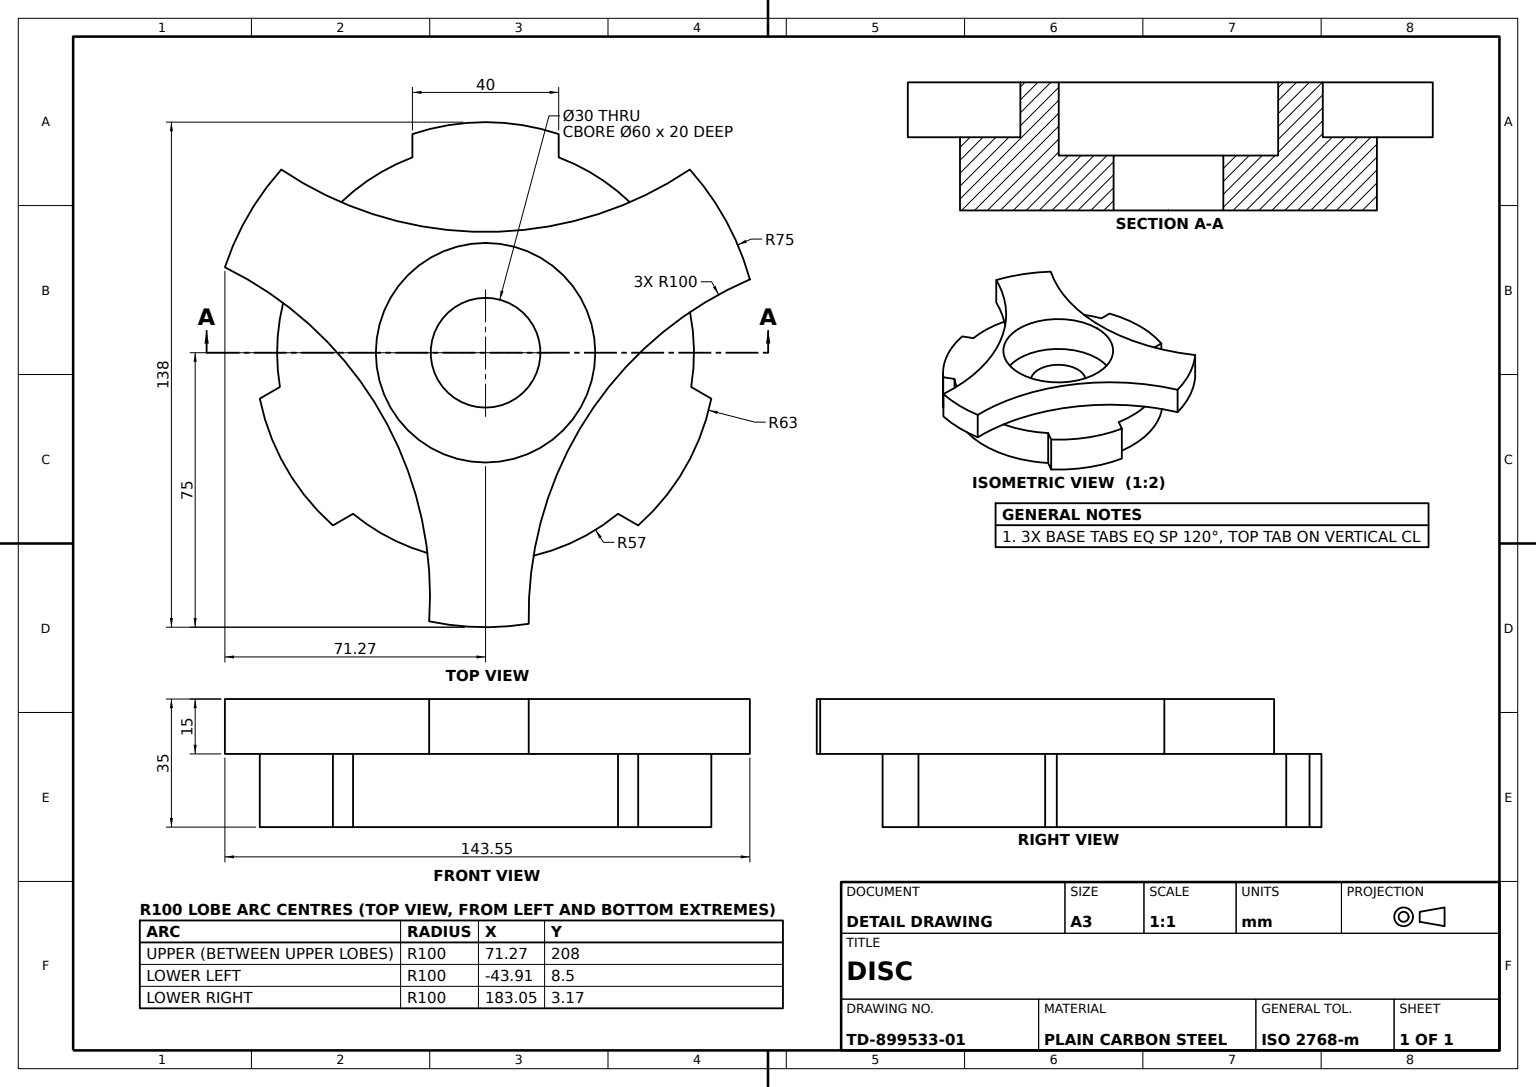
from build123d import *

# Parameters (mm, degrees)
BASE_DISC_20MM_DEPTH        = 20
THREE_LOBE_BOSS_15MM_DEPTH  = 15
COUNTERBORE_PROFILE_R       = 30
COUNTERBORE_20MM_DEEP_DEPTH = 20
THROUGH_BORE_PROFILE_R      = 15
THROUGH_BORE_DEPTH          = 107.05840812


with BuildPart() as part:
    # Base Disc Profile → Base Disc 20mm (new body)
    with BuildSketch(Plane(origin=(0, 0, 0), x_dir=(1, 0, 0), z_dir=(0, 1, 0))):
        with BuildLine():
            Line((-20, 53.37602458), (-20, 59.741108125))
            ThreePointArc((-20, 59.741108125), (0, 63), (20, 59.741108125))
            Line((20, 59.741108125), (20, 53.37602458))
            ThreePointArc((20, 53.37602458), (49.363448016, 28.5), (56.22499324, -9.367504214))
            Line((56.22499324, -9.367504214), (61.737317286, -12.550045987))
            ThreePointArc((61.737317286, -12.550045987), (54.559600438, -31.5), (41.737317286, -47.191062138))
            Line((41.737317286, -47.191062138), (36.22499324, -44.008520366))
            ThreePointArc((36.22499324, -44.008520366), (0, -57), (-36.22499324, -44.008520366))
            Line((-36.22499324, -44.008520366), (-41.737317286, -47.191062138))
            ThreePointArc((-41.737317286, -47.191062138), (-54.559600438, -31.5), (-61.737317286, -12.550045987))
            Line((-61.737317286, -12.550045987), (-56.22499324, -9.367504214))
            ThreePointArc((-56.22499324, -9.367504214), (-49.363448016, 28.5), (-20, 53.37602458))
        make_face()
    extrude(amount=BASE_DISC_20MM_DEPTH)

    # Three-Lobe Profile → Three-Lobe Boss 15mm (add)
    with BuildSketch(Plane(origin=(0, 20, 0), x_dir=(1, 0, 0), z_dir=(0, 1, 0))):
        with BuildLine():
            ThreePointArc((39.473039737, 41.120300752), (0, 33), (-39.473039737, 41.120300752))
            ThreePointArc((-39.473039737, 41.120300752), (-49.363448016, 28.5), (-55.347744931, 13.624504801))
            ThreePointArc((-55.347744931, 13.624504801), (-28.578838325, -16.5), (-15.874705194, -54.744805553))
            ThreePointArc((-15.874705194, -54.744805553), (-1.422355425, -56.98225079), (13.123625771, -55.468643815))
            ThreePointArc((13.123625771, -55.468643815), (27.648504036, -17.766556361), (55.906633869, 11.110728574))
            ThreePointArc((55.906633869, 11.110728574), (49.994641111, 27.377652568), (39.473039737, 41.120300752))
        make_face()
        with BuildLine():
            ThreePointArc((-39.473039737, 41.120300752), (-44.717521746, 43.555362101), (-49.812494678, 46.289473684))
            ThreePointArc((-49.812494678, 46.289473684), (-58.889727457, 34), (-64.994107477, 19.994148975))
            ThreePointArc((-64.994107477, 19.994148975), (-60.078810924, 16.948828776), (-55.347744931, 13.624504801))
            ThreePointArc((-55.347744931, 13.624504801), (-49.363448016, 28.5), (-39.473039737, 41.120300752))
        make_face()
        with BuildLine():
            ThreePointArc((-49.812494678, 46.289473684), (-52.867031225, 48.117274965), (-55.854579687, 50.052631579))
            ThreePointArc((-55.854579687, 50.052631579), (-64.951905284, 37.5), (-71.274140317, 23.345169137))
            ThreePointArc((-71.274140317, 23.345169137), (-68.104298093, 21.725554581), (-64.994107477, 19.994148975))
            ThreePointArc((-64.994107477, 19.994148975), (-58.889727457, 34), (-49.812494678, 46.289473684))
        make_face()
        with BuildLine():
            ThreePointArc((13.123625771, -55.468643815), (-1.422355425, -56.98225079), (-15.874705194, -54.744805553))
            ThreePointArc((-15.874705194, -54.744805553), (-15.361289177, -60.504190877), (-15.181612799, -66.283622659))
            ThreePointArc((-15.181612799, -66.283622659), (-1.676596285, -67.979327923), (11.895593178, -66.951436601))
            ThreePointArc((11.895593178, -66.951436601), (12.343713059, -61.192298339), (13.123625771, -55.468643815))
        make_face()
        with BuildLine():
            ThreePointArc((11.895593178, -66.951436601), (-1.676596285, -67.979327923), (-15.181612799, -66.283622659))
            ThreePointArc((-15.181612799, -66.283622659), (-15.237266868, -69.842829546), (-15.41956063, -73.397800716))
            ThreePointArc((-15.41956063, -73.397800716), (-1.839450143, -74.977439428), (11.801783935, -74.065632354))
            ThreePointArc((11.801783935, -74.065632354), (11.7853983, -70.507699919), (11.895593178, -66.951436601))
        make_face()
        with BuildLine():
            ThreePointArc((49.812494678, 46.289473684), (44.717521746, 43.555362101), (39.473039737, 41.120300752))
            ThreePointArc((39.473039737, 41.120300752), (49.994641111, 27.377652568), (55.906633869, 11.110728574))
            ThreePointArc((55.906633869, 11.110728574), (60.78874038, 14.198368606), (65.840986006, 16.998957666))
            ThreePointArc((65.840986006, 16.998957666), (59.652455781, 32.643292102), (49.812494678, 46.289473684))
        make_face()
        with BuildLine():
            ThreePointArc((55.854579687, 50.052631579), (52.867031225, 48.117274965), (49.812494678, 46.289473684))
            ThreePointArc((49.812494678, 46.289473684), (59.652455781, 32.643292102), (65.840986006, 16.998957666))
            ThreePointArc((65.840986006, 16.998957666), (69.029934048, 18.576855661), (72.272995877, 20.04031105))
            ThreePointArc((72.272995877, 20.04031105), (65.797824819, 35.995086458), (55.854579687, 50.052631579))
        make_face()
    extrude(amount=THREE_LOBE_BOSS_15MM_DEPTH)

    # Counterbore Profile → Counterbore 20mm Deep (cut)
    with BuildSketch(Plane(origin=(0, 35, 0), x_dir=(1, 0, 0), z_dir=(0, 1, 0))):
        with Locations(Location((0, 0, 0), (0, 0, 270))):
            Circle(COUNTERBORE_PROFILE_R)
    extrude(amount=-COUNTERBORE_20MM_DEEP_DEPTH, mode=Mode.SUBTRACT)

    # Through Bore Profile → Through Bore (cut, through all)
    with BuildSketch(Plane(origin=(0, 15, 0), x_dir=(1, 0, 0), z_dir=(0, 1, 0))):
        with Locations(Location((0, 0, 0), (0, 0, 270))):
            Circle(THROUGH_BORE_PROFILE_R)
    extrude(amount=-THROUGH_BORE_DEPTH, mode=Mode.SUBTRACT)


solid = part.part
